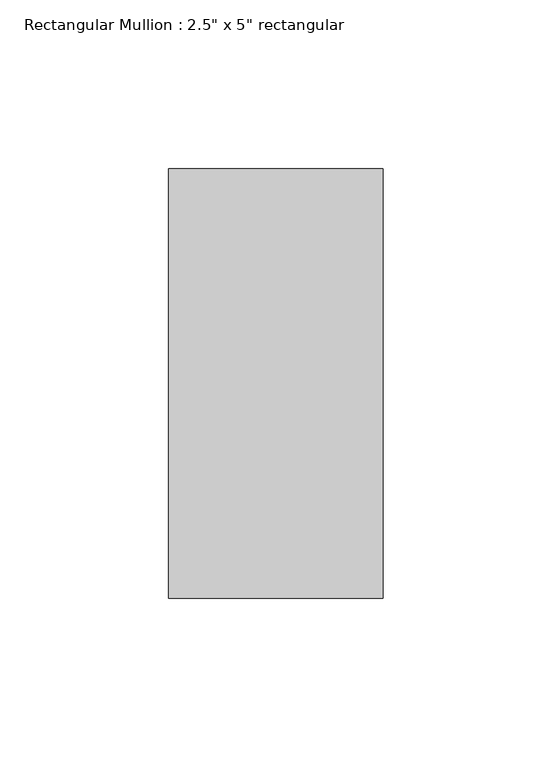
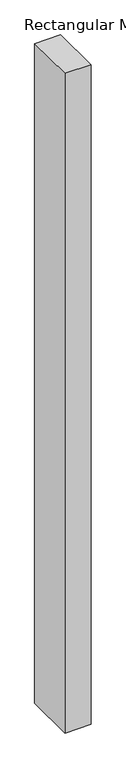
"""IFC4 building model written with IfcOpenShell, lengths in millimetres: member geometry."""

from ifc_helpers import new_model, si_unit, frame, origin, place, context, project, spatial, polyline, outline, extrude, source, transform, mapped, element, save


def member_d25e63f8(model_context):
    return source(origin(), model_context, "Body", "SweptSolid", [
        extrude(outline(polyline([(0.0, 63.5), (0.0, -63.5), (-63.5, -63.5), (-63.5, 63.5), (0.0, 63.5)])), frame((0.0, 0.0, -1697.4525236), z_axis=(0.0, 0.0, 1.0), x_axis=(1.0, 0.0, 0.0)), (0.0, 0.0, 1.0), 1697.4525236),
    ])


if __name__ == "__main__":
    model = new_model("IFC4")
    model_context = context("Model", 3, world=origin())
    ifc_project = project(units=[si_unit("LENGTHUNIT", "METRE", prefix="MILLI")], contexts=[model_context])
    site = spatial("IfcSite", under=ifc_project)
    building = spatial("IfcBuilding", under=site)
    placement = place(None, origin())
    member_shape = member_d25e63f8(model_context)
    element("IfcMember", 1, ObjectType="Rectangular Mullion : 2.5\" x 5\" rectangular", at=placement, inside=building, context=model_context, shape_type="MappedRepresentation", body=[
        mapped(member_shape, transform((0.0, 0.0, 0.0), x_axis=(1.0, 0.0, 0.0), y_axis=(0.0, 1.0, 0.0), z_axis=(0.0, 0.0, 1.0))),
    ])
    save(model, "model.ifc")

# Revit data of these elements
# Type "Rectangular Mullion : 2.5\" x 5\" rectangular"
#   built-in parameter 1007304 = 0.416667 (stored number, unit not read)
#   built-in parameter 1007301 = 0.104167 (stored number, unit not read)
#   built-in parameter 1007300 = 0.104167 (stored number, unit not read)
# Element 1 (IfcMember, "Rectangular Mullion : 2.5\" x 5\" rectangular")
#   Materials on its faces: "Aluminum"
# Materials
#   "Aluminum": class "Metal", colour RGB 247 247 247, transparency 0, Description = "Aluminum 6061", Cost = 0
